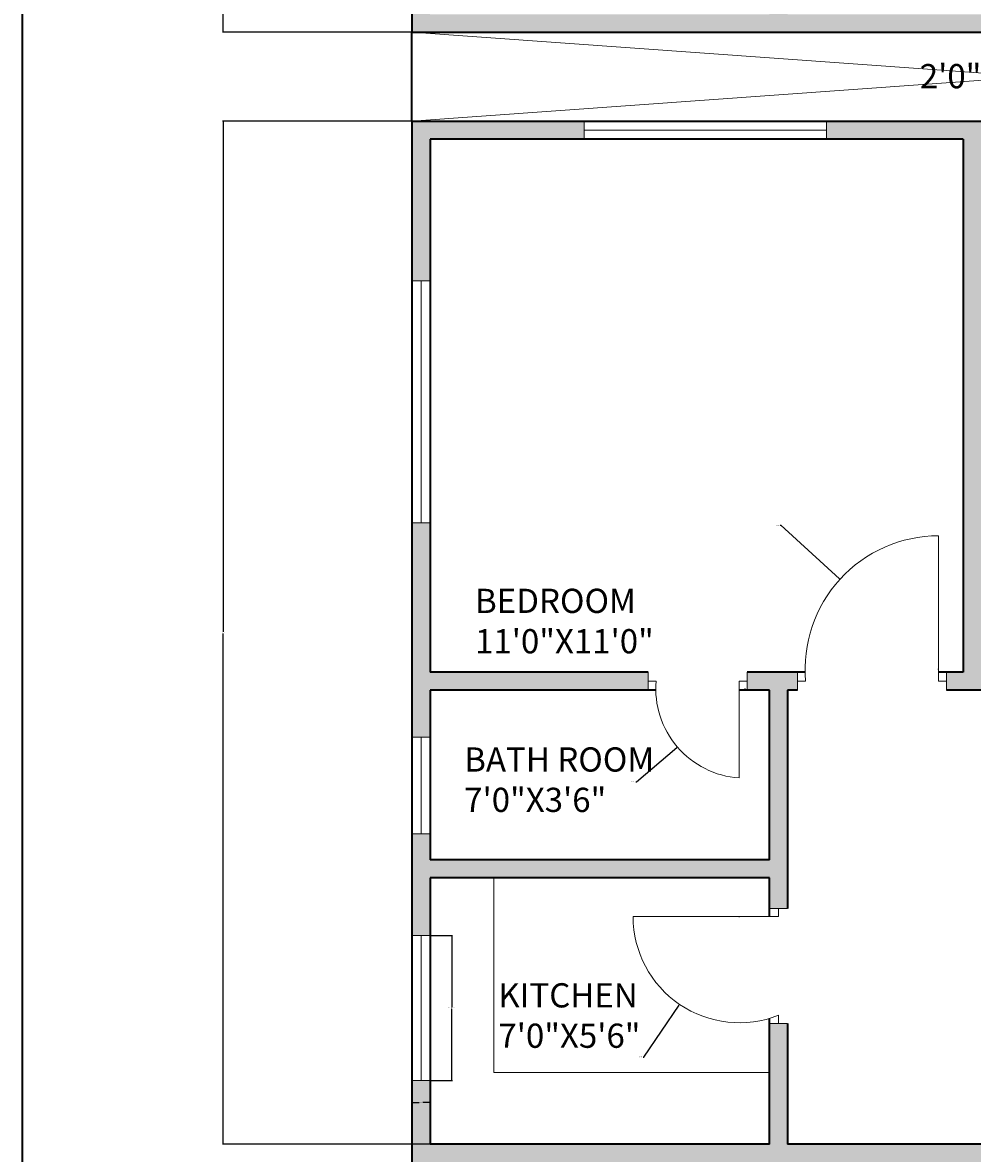
# Model space of a CAD drawing. Units: inches. Extents: x 2314 to 3223, y 1382 to 2735.
# Tile 6 of 14: x 2314 to 2549, y 1864 to 2144. Entities that reach past the tile are written whole.
import ezdxf

# ---------------------------------------------------------------- set-up
doc = ezdxf.new("R2010")
doc.units = ezdxf.units.IN
for name, color, linetype, lineweight in [('A-ANNO-DIMS', 2, 'Continuous', 18), ('A-ANNO-TTLB', 7, 'Continuous', 35), ('A-AREA-IDEN', 7, 'Continuous', 18), ('A-DOOR', 3, 'Continuous', 18), ('A-FLOR-FIXT', 8, 'Continuous', 18), ('A-FLOR-OPEN', 8, 'Continuous', 13), ('A-GLAZ', 4, 'Continuous', 18), ('A-WALL', 7, 'Continuous', 35)]:
    doc.layers.add(name, color=color, linetype=linetype, lineweight=lineweight)
doc.layers.add('A-WALL-PATT', color=251, linetype='Continuous', lineweight=13, true_color=0x636466)
doc.styles.get("Standard").update_dxf_attribs({"font": 'arial.ttf'})
doc.dimstyles.get("Standard").update_dxf_attribs({"dimtxt": 0.18, "dimasz": 0.18, "dimexe": 0.18, "dimexo": 0.0625, "dimgap": 0.09, "dimtad": 0, "dimtih": 1, "dimtoh": 1, "dimdec": 4, "dimzin": 0, "dimdsep": 46, "dimtxsty": 'Standard', "dimcen": 0.09, "dimadec": 0, "dimazin": 0, "dimtfac": 1, "dimtdec": 4, "dimtofl": 0, "dimtmove": 0, "dimatfit": 3, "dimfxl": 1, "dimtolj": 1, "dimtzin": 0, "dimarcsym": 0})

# ---------------------------------------------------------------- blocks, each defined once
blk = doc.blocks.new('WIN-PLAN-24-ALT')
for p, q in [((4.5, 24), (0, 24)), ((0, 24), (2.25, 24)), ((2.25, 24), (2.25, 0)), ((2.25, 0), (0, 0)), ((0, 0), (4.5, 0))]:
    blk.add_line(p, q)
blk = doc.blocks.new('WIN-PLAN-60')
for p, q in [((0, 4.5), (0, 0)), ((60, 2.25), (60, 4.5)), ((60, 4.5), (60, 0)), ((0, 0), (0, 2.25)), ((0, 2.25), (60, 2.25))]:
    blk.add_line(p, q)
blk = doc.blocks.new('WIN-PLAN-36')
for p, q in [((0, 36), (4.5, 36)), ((4.5, 36), (2.25, 36)), ((2.25, 36), (2.25, 0)), ((2.25, 0), (0, 0)), ((0, 0), (4.5, 0))]:
    blk.add_line(p, q)
blk = doc.blocks.new('*D15')
at = {"layer": 'A-ANNO-DIMS', "color": 0, "lineweight": -2, "transparency": 16777216}
for p, q in [((2414.96, 1918.15), (2420.47, 1918.15)), ((2420.29, 1917.97), (2420.29, 1900.33)), ((2420.29, 1882.33), (2420.29, 1899.97)), ((2414.96, 1882.15), (2420.47, 1882.15))]:
    blk.add_line(p, q, dxfattribs=at)
at = {"layer": 'A-ANNO-DIMS', "color": 0, "transparency": 16777216}
for points in [[(2420.26, 1917.97), (2420.32, 1917.97), (2420.29, 1918.15)], [(2420.26, 1882.33), (2420.32, 1882.33), (2420.29, 1882.15)]]:
    blk.add_solid(points, dxfattribs=at)
at = {"layer": 'Defpoints', "color": 0, "transparency": 16777216}
for p in [(2414.89, 1918.15), (2414.89, 1882.15), (2420.29, 1882.15)]:
    blk.add_point(p, dxfattribs=at)
at = {"layer": 'A-ANNO-DIMS', "color": 0, "transparency": 16777216, "insert": (2420.29, 1900.15), "char_height": 0.18, "attachment_point": 5}
blk.add_mtext('\\A1;WINDOW 36 TYP.', dxfattribs=at)
blk = doc.blocks.new('*D16')
at = {"layer": 'A-ANNO-DIMS', "color": 0, "lineweight": -2, "transparency": 16777216}
for p, q in [((2410.39, 1882.09), (2410.39, 1876.57)), ((2414.89, 1882.09), (2414.89, 1876.57)), ((2410.57, 1876.75), (2412.18, 1876.75)), ((2414.71, 1876.75), (2413.1, 1876.75))]:
    blk.add_line(p, q, dxfattribs=at)
at = {"layer": 'A-ANNO-DIMS', "color": 0, "transparency": 16777216}
for points in [[(2410.57, 1876.78), (2410.57, 1876.72), (2410.39, 1876.75)], [(2414.71, 1876.78), (2414.71, 1876.72), (2414.89, 1876.75)]]:
    blk.add_solid(points, dxfattribs=at)
at = {"layer": 'Defpoints', "color": 0, "transparency": 16777216}
for p in [(2410.39, 1882.15), (2414.89, 1882.15), (2410.39, 1876.75)]:
    blk.add_point(p, dxfattribs=at)
at = {"layer": 'A-ANNO-DIMS', "color": 0, "transparency": 16777216, "insert": (2412.64, 1876.75), "char_height": 0.18, "attachment_point": 5}
blk.add_mtext('\\A1;5 TYP.', dxfattribs=at)
blk = doc.blocks.new('*D33')
at = {"layer": 'A-ANNO-DIMS', "color": 0, "lineweight": -2, "transparency": 16777216}
for p, q in [((2410.33, 2119.88), (2363.51, 2119.88)), ((2363.69, 2119.7), (2363.69, 1993.32)), ((2363.69, 1866.56), (2363.69, 1992.95)), ((2414.83, 1866.38), (2363.51, 1866.38))]:
    blk.add_line(p, q, dxfattribs=at)
at = {"layer": 'A-ANNO-DIMS', "color": 0, "transparency": 16777216}
for points in [[(2363.66, 2119.7), (2363.72, 2119.7), (2363.69, 2119.88)], [(2363.66, 1866.56), (2363.72, 1866.56), (2363.69, 1866.38)]]:
    blk.add_solid(points, dxfattribs=at)
at = {"layer": 'Defpoints', "color": 0, "transparency": 16777216}
for p in [(2363.69, 2119.88), (2410.39, 2119.88), (2414.89, 1866.38)]:
    blk.add_point(p, dxfattribs=at)
at = {"layer": 'A-ANNO-DIMS', "color": 0, "transparency": 16777216, "insert": (2363.69, 1993.13), "char_height": 0.18, "attachment_point": 5}
blk.add_mtext('\\A1;253.5', dxfattribs=at)
blk = doc.blocks.new('*D34')
at = {"layer": 'A-ANNO-DIMS', "color": 0, "lineweight": -2, "transparency": 16777216}
for p, q in [((2410.33, 2381.78), (2363.51, 2381.78)), ((2363.69, 2381.6), (2363.69, 2262.02)), ((2363.69, 2142.06), (2363.69, 2261.65)), ((2410.33, 2141.88), (2363.51, 2141.88))]:
    blk.add_line(p, q, dxfattribs=at)
at = {"layer": 'A-ANNO-DIMS', "color": 0, "transparency": 16777216}
for points in [[(2363.66, 2381.6), (2363.72, 2381.6), (2363.69, 2381.78)], [(2363.66, 2142.06), (2363.72, 2142.06), (2363.69, 2141.88)]]:
    blk.add_solid(points, dxfattribs=at)
at = {"layer": 'Defpoints', "color": 0, "transparency": 16777216}
for p in [(2363.69, 2381.78), (2410.39, 2381.78), (2410.39, 2141.88)]:
    blk.add_point(p, dxfattribs=at)
at = {"layer": 'A-ANNO-DIMS', "color": 0, "transparency": 16777216, "insert": (2363.69, 2261.83), "char_height": 0.18, "attachment_point": 5}
blk.add_mtext('\\A1;239.9', dxfattribs=at)
blk = doc.blocks.new('*D65')
at = {"layer": 'A-ANNO-DIMS', "color": 0, "lineweight": -2, "transparency": 16777216}
for p, q in [((2501.56, 2019.75), (2501.74, 2019.75)), ((2501.74, 2019.75), (2516.24, 2006.51)), ((2540.66, 1984.11), (2540.84, 1984.11)), ((2540.75, 1984.02), (2540.75, 1984.2))]:
    blk.add_line(p, q, dxfattribs=at)
at = {"layer": 'A-ANNO-DIMS', "color": 0, "transparency": 16777216}
blk.add_solid([(2516.26, 2006.53), (2516.22, 2006.48), (2516.37, 2006.38)], dxfattribs=at)
at = {"layer": 'Defpoints', "color": 0, "transparency": 16777216}
for p in [(2516.37, 2006.38), (2540.75, 1984.11)]:
    blk.add_point(p, dxfattribs=at)
at = {"layer": 'A-ANNO-DIMS', "color": 0, "transparency": 16777216, "insert": (2501.08, 2019.75), "char_height": 0.18, "attachment_point": 5}
blk.add_mtext('\\A1;R33.03', dxfattribs=at)
blk = doc.blocks.new('*D78')
at = {"layer": 'A-ANNO-DIMS', "color": 0, "lineweight": -2, "transparency": 16777216}
for p, q in [((2491.35, 1922.79), (2491.53, 1922.79)), ((2491.44, 1922.7), (2491.44, 1922.88)), ((2467.81, 1887.98), (2476.57, 1900.88)), ((2467.63, 1887.98), (2467.81, 1887.98))]:
    blk.add_line(p, q, dxfattribs=at)
at = {"layer": 'A-ANNO-DIMS', "color": 0, "transparency": 16777216}
blk.add_solid([(2476.54, 1900.9), (2476.59, 1900.87), (2476.67, 1901.03)], dxfattribs=at)
at = {"layer": 'Defpoints', "color": 0, "transparency": 16777216}
for p in [(2491.44, 1922.79), (2476.67, 1901.03)]:
    blk.add_point(p, dxfattribs=at)
at = {"layer": 'A-ANNO-DIMS', "color": 0, "transparency": 16777216, "insert": (2467.08, 1887.98), "char_height": 0.18, "attachment_point": 5}
blk.add_mtext('\\A1;R26.296', dxfattribs=at)
blk = doc.blocks.new('*D84')
at = {"layer": 'A-ANNO-DIMS', "color": 0, "lineweight": -2, "transparency": 16777216}
for p, q in [((2492.81, 1979.22), (2492.99, 1979.22)), ((2492.9, 1979.13), (2492.9, 1979.31)), ((2465.98, 1956.2), (2475.94, 1964.71)), ((2465.8, 1956.2), (2465.98, 1956.2))]:
    blk.add_line(p, q, dxfattribs=at)
at = {"layer": 'A-ANNO-DIMS', "color": 0, "transparency": 16777216}
blk.add_solid([(2475.92, 1964.74), (2475.96, 1964.69), (2476.08, 1964.83)], dxfattribs=at)
at = {"layer": 'Defpoints', "color": 0, "transparency": 16777216}
for p in [(2492.9, 1979.22), (2476.08, 1964.83)]:
    blk.add_point(p, dxfattribs=at)
at = {"layer": 'A-ANNO-DIMS', "color": 0, "transparency": 16777216, "insert": (2465.25, 1956.2), "char_height": 0.18, "attachment_point": 5}
blk.add_mtext('\\A1;R22.137', dxfattribs=at)

msp = doc.modelspace()

# ---------------------------------------------------------------- hatches: boundary and pattern name
at = {"layer": 'A-WALL-PATT'}
h = msp.add_hatch(color=256, dxfattribs=at)
h.dxf.hatch_style = 1
h.paths.add_polyline_path([(2443.3302, 2379.5332), (2443.3302, 2381.7832), (2410.3927, 2381.7832), (2410.3927, 2336.7008), (2414.8927, 2336.7008), (2414.8927, 2377.2832), (2443.3302, 2377.2832)])
h.paths.add_polyline_path([(2561.3645, 2379.5332), (2561.3645, 2381.7832), (2503.3302, 2381.7832), (2503.3302, 2377.2832), (2546.8927, 2377.2832), (2546.8927, 2245.2832), (2541.8787, 2245.2832), (2541.8787, 2240.7832), (2551.3927, 2240.7832), (2551.3927, 2377.2832), (2561.3645, 2377.2832)])
h.paths.add_polyline_path([(2656.0607, 2381.7832), (2597.3645, 2381.7832), (2597.3645, 2377.2832), (2617.3927, 2377.2832), (2617.3927, 2257.2832), (2584.2532, 2257.2832), (2584.2532, 2252.7832), (2625.8528, 2252.7832), (2625.8528, 2255.0332), (2625.8528, 2257.2832), (2621.8927, 2257.2832), (2621.8927, 2377.2832), (2656.0607, 2377.2832), (2656.0607, 2379.5332)])
h.paths.add_polyline_path([(2807.3418, 2381.7832), (2716.0607, 2381.7832), (2716.0607, 2377.2832), (2765.8927, 2377.2832), (2765.8927, 2257.2832), (2661.6935, 2257.2832), (2661.6935, 2252.7832), (2765.8927, 2252.7832), (2765.8927, 2146.2832), (2760.9259, 2146.2832), (2760.9259, 2141.8832), (2775.7119, 2141.8832), (2775.7119, 2146.2832), (2770.3927, 2146.2832), (2770.3927, 2252.7832), (2877.684, 2252.7832), (2877.684, 2255.0332), (2877.684, 2257.2832), (2770.3927, 2257.2832), (2770.3927, 2377.2832), (2807.3418, 2377.2832), (2807.3418, 2379.5332)])
h.paths.add_polyline_path([(2937.2118, 2381.7832), (2867.3418, 2381.7832), (2867.3418, 2377.2832), (2914.3927, 2377.2832), (2914.3927, 2257.2832), (2908.4124, 2257.2832), (2908.4124, 2252.7832), (2960.6432, 2252.7832), (2960.6432, 2255.0332), (2960.6432, 2257.2832), (2918.8927, 2257.2832), (2918.8927, 2377.2832), (2937.2118, 2377.2832)])
h.paths.add_polyline_path([(3022.1601, 2381.7832), (2973.2118, 2381.7832), (2973.2118, 2379.5332), (2973.2118, 2377.2832), (2984.8927, 2377.2832), (2984.8927, 2257.2832), (2980.0601, 2257.2832), (2980.0601, 2252.7832), (2984.8927, 2252.7832), (2984.8927, 2240.7832), (2995.668, 2240.7832), (2995.668, 2243.0332), (2995.668, 2245.2832), (2989.3927, 2245.2832), (2989.3927, 2377.2832), (3022.1601, 2377.2832), (3022.1601, 2379.5332)])
h.paths.add_polyline_path([(3125.8927, 2381.7832), (3082.1601, 2381.7832), (3082.1601, 2377.2832), (3121.3927, 2377.2832), (3121.3927, 2334.7388), (3125.8927, 2334.7388)])
h.paths.add_polyline_path([(3125.8927, 2274.7388), (3121.3927, 2274.7388), (3121.3927, 2245.2832), (3066.4832, 2245.2832), (3066.4832, 2240.7832), (3121.3927, 2240.7832), (3121.3927, 2232.1868), (3125.8927, 2232.1868)])
h.paths.add_polyline_path([(3125.8927, 2208.1868), (3121.3927, 2208.1868), (3121.3927, 2198.7832), (3037.3927, 2198.7832), (3037.3927, 2240.7832), (3041.2694, 2240.7832), (3041.2694, 2243.0332), (3041.2694, 2245.2832), (3026.8205, 2245.2832), (3026.8205, 2240.7832), (3032.8927, 2240.7832), (3032.8927, 2190.4022), (3037.3927, 2190.4022), (3037.3927, 2194.2832), (3121.3927, 2194.2832), (3121.3927, 2182.1835), (3125.8927, 2182.1835)])
h.paths.add_polyline_path([(3125.8927, 2158.1835), (3121.3927, 2158.1835), (3121.3927, 2146.2832), (3037.3927, 2146.2832), (3037.3927, 2169.3726), (3035.1427, 2169.3726), (3032.8927, 2169.3726), (3032.8927, 2146.2832), (2812.7301, 2146.2832), (2812.7301, 2144.0832), (2812.7301, 2141.8832), (2818.3927, 2141.8832), (2818.3927, 1970.1316), (2822.8927, 1970.1316), (2822.8927, 1978.8832), (2903.9846, 1978.8832), (2903.9846, 1981.1332), (2903.9846, 1983.3832), (2822.8927, 1983.3832), (2822.8927, 2115.3832), (2851.7162, 2115.3832), (2851.7162, 2117.6332), (2851.7162, 2119.8832), (2822.8927, 2119.8832), (2822.8927, 2141.8832), (3125.8927, 2141.8832)])
h.paths.add_polyline_path([(3125.8927, 2119.8832), (3081.193, 2119.8832), (3081.193, 2115.3832), (3121.3927, 2115.3832), (3121.3927, 2071.8188), (3125.8927, 2071.8188)], flags=17)
h.paths.add_polyline_path([(2989.3927, 2115.3832), (3021.193, 2115.3832), (3021.193, 2117.6332), (3021.193, 2119.8832), (2979.123, 2119.8832), (2979.123, 2115.3832), (2984.8927, 2115.3832), (2984.8927, 2019.3832), (2981.9225, 2019.3832), (2981.9225, 2014.8832), (2984.8927, 2014.8832), (2984.8927, 1983.3832), (2984.8927, 1978.8832), (2989.3927, 1978.8832), (2989.3927, 1983.3832)], flags=17)
h.paths.add_polyline_path([(2947.3927, 2115.3832), (2955.123, 2115.3832), (2955.123, 2117.6332), (2955.123, 2119.8832), (2911.7162, 2119.8832), (2911.7162, 2115.3832), (2942.8927, 2115.3832), (2942.8927, 1983.3832), (2936.7017, 1983.3832), (2936.7017, 1978.8832), (2947.3927, 1978.8832), (2947.3927, 1983.3832), (2947.3927, 2014.8832), (2960.7167, 2014.8832), (2960.7167, 2017.1332), (2960.7167, 2019.3832), (2947.3927, 2019.3832)], flags=17)
h.paths.add_polyline_path([(3037.3927, 1978.8832), (3041.8276, 1978.8832), (3041.8276, 1981.1332), (3041.8276, 1983.3832), (3025.477, 1983.3832), (3025.477, 1978.8832), (3032.8927, 1978.8832), (3032.8927, 1927.1259), (3035.1427, 1927.1259), (3037.3927, 1927.1259)])
h.paths.add_polyline_path([(3125.8927, 2011.8188), (3123.6427, 2011.8188), (3121.3927, 2011.8188), (3121.3927, 1983.3832), (3065, 1983.3832), (3065, 1978.8832), (3121.3927, 1978.8832), (3121.3927, 1970.5932), (3125.8927, 1970.5932)], flags=17)
h.paths.add_polyline_path([(2994.2341, 1983.3832), (2989.3927, 1983.3832), (2989.3927, 1978.8832), (2994.2341, 1978.8832), (2994.2341, 1981.1332)], flags=16)
h.paths.add_polyline_path([(3125.8927, 1946.5932), (3121.3927, 1946.5932), (3121.3927, 1936.8832), (3037.3927, 1936.8832), (3037.3927, 1932.3832), (3121.3927, 1932.3832), (3121.3927, 1919.825), (3125.8927, 1919.825)])
h.paths.add_polyline_path([(3125.8927, 1883.825), (3121.3927, 1883.825), (3121.3927, 1866.3832), (3037.3927, 1866.3832), (3037.3927, 1899.0954), (3035.1427, 1899.0954), (3032.8927, 1899.0954), (3032.8927, 1866.3832), (2822.8927, 1866.3832), (2822.8927, 1938.7212), (2820.6427, 1938.7212), (2818.3927, 1938.7212), (2818.3927, 1786.9239), (2822.8927, 1786.9239), (2822.8927, 1861.8832), (3032.8927, 1861.8832), (3032.8927, 1825.1023), (3037.3927, 1825.1023), (3037.3927, 1861.8832), (3121.3927, 1861.8832), (3121.3927, 1844.6765), (3125.8927, 1844.6765)])
h.paths.add_polyline_path([(3125.8927, 1808.6765), (3121.3927, 1808.6765), (3121.3927, 1795.8832), (3037.3927, 1795.8832), (3037.3927, 1799.4755), (3032.8927, 1799.4755), (3032.8927, 1749.3832), (3026.5034, 1749.3832), (3026.5034, 1744.8832), (3032.8927, 1744.8832), (3034.9255, 1744.8832), (3043.1326, 1744.8832), (3043.1326, 1747.1332), (3043.1326, 1749.3832), (3037.3927, 1749.3832), (3037.3927, 1791.3832), (3121.3927, 1791.3832), (3121.3927, 1783.3103), (3125.8927, 1783.3103)])
h.paths.add_polyline_path([(3125.8927, 1759.3103), (3121.3927, 1759.3103), (3121.3927, 1749.3832), (3065.1845, 1749.3832), (3065.1845, 1744.8832), (3121.3927, 1744.8832), (3121.3927, 1709.3573), (3125.8927, 1709.3573)])
h.paths.add_polyline_path([(3125.8927, 1649.3573), (3121.3927, 1649.3573), (3121.3927, 1612.8832), (3095.116, 1612.8832), (3095.116, 1608.3832), (3125.8927, 1608.3832)])
h.paths.add_polyline_path([(3035.116, 1612.8832), (2993.8927, 1612.8832), (2993.8927, 1744.8832), (2998.7409, 1744.8832), (2998.7409, 1749.3832), (2989.3927, 1749.3832), (2989.3927, 1744.8832), (2989.3927, 1701.3832), (2972.8226, 1701.3832), (2972.8226, 1696.8832), (2989.3927, 1696.8832), (2989.3927, 1612.8832), (2978.2225, 1612.8832), (2978.2225, 1608.3832), (3035.116, 1608.3832), (3035.116, 1610.6332)])
h.paths.add_polyline_path([(2947.3927, 1696.8832), (2950.7566, 1696.8832), (2950.7566, 1699.1332), (2950.7566, 1701.3832), (2947.3927, 1701.3832), (2947.3927, 1744.8832), (2947.3927, 1749.3832), (2937.649, 1749.3832), (2937.649, 1744.8832), (2942.8927, 1744.8832), (2942.8927, 1612.8832), (2907.783, 1612.8832), (2907.783, 1608.3832), (2954.2225, 1608.3832), (2954.2225, 1610.6332), (2954.2225, 1612.8832), (2947.3927, 1612.8832)])
h.paths.add_polyline_path([(2822.8927, 1744.8832), (2905.3491, 1744.8832), (2905.3491, 1747.1332), (2905.3491, 1749.3832), (2822.8927, 1749.3832), (2822.8927, 1756.9185), (2818.3927, 1756.9185), (2818.3927, 1612.8832), (2818.3927, 1569.1205), (2722.3927, 1569.1205), (2722.3927, 1612.8832), (2722.3927, 1756.9185), (2717.8927, 1756.9185), (2717.8927, 1750.0143), (2633.6297, 1750.0143), (2633.6437, 1745.2665), (2717.8927, 1745.5143), (2717.8927, 1612.8832), (2689.8467, 1612.8832), (2689.8467, 1608.3832), (2717.8927, 1608.3832), (2717.8927, 1564.6205), (2722.3927, 1564.6205), (2822.8927, 1564.6205), (2822.8927, 1569.1205), (2822.8927, 1608.3832), (2847.783, 1608.3832), (2847.783, 1610.6332), (2847.783, 1612.8832), (2822.8927, 1612.8832)])
h.paths.add_polyline_path([(2629.8467, 1612.8832), (2597.8927, 1612.8832), (2597.8927, 1744.8832), (2597.8927, 1745.1613), (2601.5887, 1745.1721), (2601.5816, 1747.5932), (2601.5745, 1750.0143), (2593.3927, 1750.0143), (2593.3927, 1744.8832), (2593.3927, 1713.3832), (2589.7588, 1713.3832), (2589.7588, 1708.8832), (2593.3927, 1708.8832), (2593.3927, 1612.8832), (2582.3793, 1612.8832), (2582.3793, 1608.3832), (2629.8467, 1608.3832), (2629.8467, 1610.6332)])
h.paths.add_polyline_path([(2551.3927, 1708.8832), (2567.6776, 1708.8832), (2567.6776, 1711.1332), (2567.6776, 1713.3832), (2551.3927, 1713.3832), (2551.3927, 1744.8832), (2551.3927, 1750.0143), (2543.5657, 1750.0143), (2543.5657, 1747.5079), (2543.5657, 1745.0014), (2546.8927, 1745.0112), (2546.8927, 1744.8832), (2546.8927, 1612.8832), (2502.9339, 1612.8832), (2502.9339, 1608.3832), (2558.3793, 1608.3832), (2558.3793, 1610.6332), (2558.3793, 1612.8832), (2551.3927, 1612.8832)])
h.paths.add_polyline_path([(2414.8927, 1656.2547), (2410.3927, 1656.2547), (2410.3927, 1608.3832), (2442.9339, 1608.3832), (2442.9339, 1610.6332), (2442.9339, 1612.8832), (2414.8927, 1612.8832)])
h.paths.add_polyline_path([(2414.8927, 1744.8832), (2468.8906, 1744.8832), (2468.8906, 1747.1332), (2468.8906, 1749.3832), (2414.8927, 1749.3832), (2414.8927, 1757.7622), (2410.3927, 1757.7622), (2410.3927, 1716.2547), (2414.8927, 1716.2547)])
h.paths.add_polyline_path([(2414.8927, 1791.3832), (2498.8927, 1791.3832), (2498.8927, 1749.3832), (2492.9799, 1749.3832), (2492.9799, 1744.8832), (2498.8927, 1744.8832), (2503.3927, 1744.8832), (2508.0135, 1744.8968), (2508.0059, 1747.4556), (2507.9984, 1750.0143), (2503.3927, 1750.0143), (2503.3927, 1802.6362), (2501.1427, 1802.6362), (2498.8927, 1802.6362), (2498.8927, 1795.8832), (2414.8927, 1795.8832), (2414.8927, 1808.0943), (2410.3927, 1808.0943), (2410.3927, 1781.7622), (2414.8927, 1781.7622)])
h.paths.add_polyline_path([(2722.3927, 1937.589), (2720.1427, 1937.589), (2717.8927, 1937.589), (2717.8927, 1866.3832), (2503.3927, 1866.3832), (2503.3927, 1896.3484), (2498.8927, 1896.3484), (2498.8927, 1866.3832), (2414.8927, 1866.3832), (2414.8927, 1882.1496), (2410.3927, 1882.1496), (2410.3927, 1844.0943), (2414.8927, 1844.0943), (2414.8927, 1861.8832), (2498.8927, 1861.8832), (2498.8927, 1831.4783), (2501.1427, 1831.4783), (2503.3927, 1831.4783), (2503.3927, 1861.8832), (2717.8927, 1861.8832), (2717.8927, 1786.9239), (2722.3927, 1786.9239)])
h.paths.add_polyline_path([(2414.8927, 1932.3832), (2498.8927, 1932.3832), (2498.8927, 1924.7883), (2503.3927, 1924.7883), (2503.3927, 1978.8832), (2505.8599, 1978.8832), (2505.8599, 1981.1332), (2505.8599, 1983.3832), (2493.3697, 1983.3832), (2493.3697, 1978.8832), (2498.8927, 1978.8832), (2498.8927, 1936.8832), (2414.8927, 1936.8832), (2414.8927, 1943.2834), (2410.3927, 1943.2834), (2410.3927, 1918.1496), (2414.8927, 1918.1496)])
h.paths.add_polyline_path([(2414.8927, 2020.3133), (2412.6427, 2020.3133), (2410.3927, 2020.3133), (2410.3927, 1967.2834), (2414.8927, 1967.2834), (2414.8927, 1978.8832), (2468.8513, 1978.8832), (2468.8513, 1981.1332), (2468.8513, 1983.3832), (2414.8927, 1983.3832)])
h.paths.add_polyline_path([(2414.8927, 2115.3832), (2453.004, 2115.3832), (2453.004, 2117.6332), (2453.004, 2119.8832), (2410.3927, 2119.8832), (2410.3927, 2080.3133), (2414.8927, 2080.3133)], flags=17)
h.paths.add_polyline_path([(2559.0969, 2117.6332), (2559.0969, 2119.8832), (2513.004, 2119.8832), (2513.004, 2115.3832), (2546.8927, 2115.3832), (2546.8927, 1983.3832), (2542.7531, 1983.3832), (2542.7531, 1978.8832), (2551.3927, 1978.8832), (2551.3927, 2014.8832), (2570.3098, 2014.8832), (2570.3098, 2017.1332), (2570.3098, 2019.3832), (2551.3927, 2019.3832), (2551.3927, 2115.3832), (2559.0969, 2115.3832)], flags=17)
h.paths.add_polyline_path([(2628.5073, 2117.6332), (2628.5073, 2119.8832), (2583.0969, 2119.8832), (2583.0969, 2115.3832), (2593.3927, 2115.3832), (2593.3927, 2019.3832), (2590.2108, 2019.3832), (2590.2108, 2014.8832), (2593.3927, 2014.8832), (2593.3927, 1978.8832), (2601.5907, 1978.8832), (2601.5907, 1981.1332), (2601.5907, 1983.3832), (2597.8927, 1983.3832), (2597.8927, 2115.3832), (2628.5073, 2115.3832)], flags=17)
h.paths.add_polyline_path([(2722.3927, 2141.8832), (2726.9871, 2141.8832), (2726.9871, 2144.2705), (2726.9871, 2146.2832), (2503.3927, 2146.2832), (2503.3927, 2168.2161), (2501.1427, 2168.2161), (2498.8927, 2168.2161), (2498.8927, 2146.2832), (2414.8927, 2146.2832), (2414.8927, 2156.5041), (2410.3927, 2156.5041), (2410.3927, 2141.8832), (2717.8927, 2141.8832), (2717.8927, 2119.8832), (2688.5073, 2119.8832), (2688.5073, 2115.3832), (2717.8927, 2115.3832), (2717.8927, 1983.3832), (2633.2454, 1983.3832), (2633.2454, 1978.8832), (2717.8927, 1978.8832), (2717.8927, 1970.1316), (2720.1427, 1970.1316), (2722.3927, 1970.1316)])
h.paths.add_polyline_path([(2557.3704, 1462.9278), (2940.0934, 1462.9278), (2940.0934, 1512.3848), (2557.3704, 1512.3848)], flags=9)
h.paths.add_polyline_path([(2846.2527, 1703.1384), (2892.8612, 1703.1384), (2892.8612, 1725.5272), (2846.2527, 1725.5272)], flags=25)
h.paths.add_polyline_path([(2885.6102, 1812.1147), (2946.1505, 1812.1147), (2946.1505, 1834.5035), (2885.6102, 1834.5035)], flags=25)
h.paths.add_polyline_path([(2885.6102, 1884.183), (2946.1505, 1884.183), (2946.1505, 1906.5718), (2885.6102, 1906.5718)], flags=25)
h.paths.add_polyline_path([(3066.365, 1705.5431), (3112.9735, 1705.5431), (3112.9735, 1727.9319), (3066.365, 1727.9319)], flags=9)
h.paths.add_polyline_path([(3061.8255, 1887.7513), (3101.6154, 1887.7513), (3101.6154, 1910.1401), (3061.8255, 1910.1401)], flags=25)
h.paths.add_polyline_path([(3063.3679, 1816.2121), (3103.1578, 1816.2121), (3103.1578, 1838.6009), (3063.3679, 1838.6009)], flags=25)
h.paths.add_polyline_path([(3053.3743, 1768.416), (3107.1329, 1768.416), (3107.1329, 1790.8048), (3053.3743, 1790.8048)], flags=25)
h.paths.add_polyline_path([(3061.6068, 1943.822), (3115.3653, 1943.822), (3115.3653, 1966.2109), (3061.6068, 1966.2109)], flags=9)
h.paths.add_polyline_path([(2745.0978, 1763.6604), (2797.9354, 1763.6604), (2797.9354, 1776.0247), (2745.0978, 1776.0247)], flags=9)
h.paths.add_polyline_path([(2574.2135, 1819.2586), (2634.7538, 1819.2586), (2634.7538, 1841.6474), (2574.2135, 1841.6474)], flags=25)
h.paths.add_polyline_path([(2574.2135, 1891.3269), (2634.7538, 1891.3269), (2634.7538, 1913.7157), (2574.2135, 1913.7157)], flags=25)
h.paths.add_polyline_path([(2638.4466, 1702.43), (2685.0551, 1702.43), (2685.0551, 1724.8188), (2638.4466, 1724.8188)], flags=25)
h.paths.add_polyline_path([(2435.9715, 1697.1215), (2482.5799, 1697.1215), (2482.5799, 1719.5103), (2435.9715, 1719.5103)], flags=9)
h.paths.add_polyline_path([(2431.2046, 1893.7833), (2470.9945, 1893.7833), (2470.9945, 1916.1721), (2431.2046, 1916.1721)], flags=25)
h.paths.add_polyline_path([(2439.8144, 1817.2116), (2479.6043, 1817.2116), (2479.6043, 1839.6004), (2439.8144, 1839.6004)], flags=25)
h.paths.add_polyline_path([(2441.2607, 1753.0942), (2495.0192, 1753.0942), (2495.0192, 1775.483), (2441.2607, 1775.483)], flags=25)
h.paths.add_polyline_path([(2421.216, 1945.3109), (2474.9746, 1945.3109), (2474.9746, 1967.6997), (2421.216, 1967.6997)], flags=25)
h.paths.add_polyline_path([(2585.4464, 1627.5703), (2585.4464, 1679), (2563.0576, 1679), (2563.0576, 1627.5703)], flags=9)
h.paths.add_polyline_path([(2978.3497, 1618.7039), (2978.3497, 1670.1337), (2955.9609, 1670.1337), (2955.9609, 1618.7039)], flags=9)
h.paths.add_polyline_path([(2975.9502, 2041.7828), (2975.9502, 2093.2125), (2953.5614, 2093.2125), (2953.5614, 2041.7828)], flags=25)
h.paths.add_polyline_path([(2835.6537, 1989.2068), (2882.2621, 1989.2068), (2882.2621, 2011.5956), (2835.6537, 2011.5956)], flags=25)
h.paths.add_polyline_path([(2649.3769, 1997.5659), (2695.9853, 1997.5659), (2695.9853, 2019.9547), (2649.3769, 2019.9547)], flags=25)
h.paths.add_polyline_path([(2579.9087, 2040.3429), (2579.9087, 2091.7726), (2557.5198, 2091.7726), (2557.5198, 2040.3429)], flags=25)
h.paths.add_polyline_path([(2783.2404, 1883.1956), (2783.2404, 2067.1369), (2764.694, 2067.1369), (2764.694, 1883.1956)], flags=9)
h.paths.add_polyline_path([(3055.8435, 1993.5571), (3102.4519, 1993.5571), (3102.4519, 2015.9459), (3055.8435, 2015.9459)], flags=25)
h.paths.add_polyline_path([(2423.6009, 1984.6082), (2470.2094, 1984.6082), (2470.2094, 2006.997), (2423.6009, 2006.997)], flags=25)
h.paths.add_polyline_path([(2973.4115, 2123.1668), (3013.1319, 2123.1668), (3013.1319, 2135.531), (2973.4115, 2135.531)], flags=25)
h.paths.add_polyline_path([(2534.3846, 2124.6231), (2574.105, 2124.6231), (2574.105, 2136.9874), (2534.3846, 2136.9874)], flags=25)
h.paths.add_polyline_path([(2829.1368, 2188.1931), (2889.411, 2188.1931), (2889.411, 2210.5819), (2829.1368, 2210.5819)], flags=9)
h.paths.add_polyline_path([(2633.2547, 2185.0437), (2693.5289, 2185.0437), (2693.5289, 2207.4325), (2633.2547, 2207.4325)], flags=9)
h.paths.add_polyline_path([(2445.1812, 2167.0395), (2496.611, 2167.0395), (2496.611, 2189.4284), (2445.1812, 2189.4284)], flags=9)
h.paths.add_polyline_path([(2429.1678, 2194.5482), (2480.5975, 2194.5482), (2480.5975, 2216.937), (2429.1678, 2216.937)], flags=9)
h.paths.add_polyline_path([(3060.1138, 2158.1056), (3111.5436, 2158.1056), (3111.5436, 2180.4944), (3060.1138, 2180.4944)], flags=9)
h.paths.add_polyline_path([(3055.6824, 2201.2631), (3107.1122, 2201.2631), (3107.1122, 2223.652), (3055.6824, 2223.652)], flags=25)
h.paths.add_polyline_path([(3044.3482, 2257.7345), (3090.9567, 2257.7345), (3090.9567, 2280.1233), (3044.3482, 2280.1233)], flags=9)
h.paths.add_polyline_path([(2942.5437, 2306.9625), (2982.3336, 2306.9625), (2982.3336, 2329.3513), (2942.5437, 2329.3513)], flags=9)
h.paths.add_polyline_path([(2799.5865, 2259.1663), (2846.195, 2259.1663), (2846.195, 2281.5551), (2799.5865, 2281.5551)], flags=25)
h.paths.add_polyline_path([(2670.4998, 2261.1493), (2717.1082, 2261.1493), (2717.1082, 2283.5381), (2670.4998, 2283.5381)], flags=25)
h.paths.add_polyline_path([(2553.0333, 2302.7735), (2592.8232, 2302.7735), (2592.8232, 2325.1624), (2553.0333, 2325.1624)], flags=9)
h.paths.add_polyline_path([(2432.0288, 2268.6489), (2478.6372, 2268.6489), (2478.6372, 2291.0377), (2432.0288, 2291.0377)], flags=9)
h = msp.add_hatch(color=256, dxfattribs=at)
h.dxf.hatch_style = 1
h.paths.add_polyline_path([(2503.3927, 2240.7832), (2507.7952, 2240.7832), (2507.7952, 2245.2832), (2496.4262, 2245.2832), (2496.4262, 2243.0332), (2496.4262, 2240.7832), (2498.8927, 2240.7832), (2498.8927, 2198.7832), (2414.8927, 2198.7832), (2414.8927, 2206.5718), (2410.3927, 2206.5718), (2410.3927, 2180.5041), (2412.6427, 2180.5041), (2414.8927, 2180.5041), (2414.8927, 2194.2832), (2498.8927, 2194.2832), (2498.8927, 2191.0069), (2503.3927, 2191.0069)])
h.paths.add_polyline_path([(2414.8927, 2276.7008), (2410.3927, 2276.7008), (2410.3927, 2230.5718), (2414.8927, 2230.5718), (2414.8927, 2240.7832), (2474.2564, 2240.7832), (2474.2564, 2243.0332), (2474.2564, 2245.2832), (2414.8927, 2245.2832)])
h.paths.add_polyline_path([(2557.3704, 1462.9278), (2940.0934, 1462.9278), (2940.0934, 1512.3848), (2557.3704, 1512.3848)], flags=9)
h.paths.add_polyline_path([(2846.2527, 1703.1384), (2892.8612, 1703.1384), (2892.8612, 1725.5272), (2846.2527, 1725.5272)], flags=9)
h.paths.add_polyline_path([(2885.6102, 1812.1147), (2946.1505, 1812.1147), (2946.1505, 1834.5035), (2885.6102, 1834.5035)], flags=9)
h.paths.add_polyline_path([(2885.6102, 1884.183), (2946.1505, 1884.183), (2946.1505, 1906.5718), (2885.6102, 1906.5718)], flags=9)
h.paths.add_polyline_path([(3066.365, 1705.5431), (3112.9735, 1705.5431), (3112.9735, 1727.9319), (3066.365, 1727.9319)], flags=9)
h.paths.add_polyline_path([(3061.8255, 1887.7513), (3101.6154, 1887.7513), (3101.6154, 1910.1401), (3061.8255, 1910.1401)], flags=9)
h.paths.add_polyline_path([(3063.3679, 1816.2121), (3103.1578, 1816.2121), (3103.1578, 1838.6009), (3063.3679, 1838.6009)], flags=9)
h.paths.add_polyline_path([(3053.3743, 1768.416), (3107.1329, 1768.416), (3107.1329, 1790.8048), (3053.3743, 1790.8048)], flags=9)
h.paths.add_polyline_path([(3061.6068, 1943.822), (3115.3653, 1943.822), (3115.3653, 1966.2109), (3061.6068, 1966.2109)], flags=9)
h.paths.add_polyline_path([(2745.0978, 1763.6604), (2797.9354, 1763.6604), (2797.9354, 1776.0247), (2745.0978, 1776.0247)], flags=9)
h.paths.add_polyline_path([(2574.2135, 1819.2586), (2634.7538, 1819.2586), (2634.7538, 1841.6474), (2574.2135, 1841.6474)], flags=9)
h.paths.add_polyline_path([(2574.2135, 1891.3269), (2634.7538, 1891.3269), (2634.7538, 1913.7157), (2574.2135, 1913.7157)], flags=9)
h.paths.add_polyline_path([(2638.4466, 1702.43), (2685.0551, 1702.43), (2685.0551, 1724.8188), (2638.4466, 1724.8188)], flags=9)
h.paths.add_polyline_path([(2435.9715, 1697.1215), (2482.5799, 1697.1215), (2482.5799, 1719.5103), (2435.9715, 1719.5103)], flags=9)
h.paths.add_polyline_path([(2431.2046, 1893.7833), (2470.9945, 1893.7833), (2470.9945, 1916.1721), (2431.2046, 1916.1721)], flags=9)
h.paths.add_polyline_path([(2439.8144, 1817.2116), (2479.6043, 1817.2116), (2479.6043, 1839.6004), (2439.8144, 1839.6004)], flags=9)
h.paths.add_polyline_path([(2441.2607, 1753.0942), (2495.0192, 1753.0942), (2495.0192, 1775.483), (2441.2607, 1775.483)], flags=9)
h.paths.add_polyline_path([(2421.216, 1945.3109), (2474.9746, 1945.3109), (2474.9746, 1967.6997), (2421.216, 1967.6997)], flags=9)
h.paths.add_polyline_path([(2585.4464, 1627.5703), (2585.4464, 1679), (2563.0576, 1679), (2563.0576, 1627.5703)], flags=9)
h.paths.add_polyline_path([(2978.3497, 1618.7039), (2978.3497, 1670.1337), (2955.9609, 1670.1337), (2955.9609, 1618.7039)], flags=9)
h.paths.add_polyline_path([(2975.9502, 2041.7828), (2975.9502, 2093.2125), (2953.5614, 2093.2125), (2953.5614, 2041.7828)], flags=9)
h.paths.add_polyline_path([(2835.6537, 1989.2068), (2882.2621, 1989.2068), (2882.2621, 2011.5956), (2835.6537, 2011.5956)], flags=9)
h.paths.add_polyline_path([(2649.3769, 1997.5659), (2695.9853, 1997.5659), (2695.9853, 2019.9547), (2649.3769, 2019.9547)], flags=9)
h.paths.add_polyline_path([(2579.9087, 2040.3429), (2579.9087, 2091.7726), (2557.5198, 2091.7726), (2557.5198, 2040.3429)], flags=9)
h.paths.add_polyline_path([(2783.2404, 1883.1956), (2783.2404, 2067.1369), (2764.694, 2067.1369), (2764.694, 1883.1956)], flags=9)
h.paths.add_polyline_path([(3055.8435, 1993.5571), (3102.4519, 1993.5571), (3102.4519, 2015.9459), (3055.8435, 2015.9459)], flags=9)
h.paths.add_polyline_path([(2423.6009, 1984.6082), (2470.2094, 1984.6082), (2470.2094, 2006.997), (2423.6009, 2006.997)], flags=9)
h.paths.add_polyline_path([(2973.4115, 2123.1668), (3013.1319, 2123.1668), (3013.1319, 2135.531), (2973.4115, 2135.531)], flags=9)
h.paths.add_polyline_path([(2534.3846, 2124.6231), (2574.105, 2124.6231), (2574.105, 2136.9874), (2534.3846, 2136.9874)], flags=9)
h.paths.add_polyline_path([(2829.1368, 2188.1931), (2889.411, 2188.1931), (2889.411, 2210.5819), (2829.1368, 2210.5819)], flags=9)
h.paths.add_polyline_path([(2633.2547, 2185.0437), (2693.5289, 2185.0437), (2693.5289, 2207.4325), (2633.2547, 2207.4325)], flags=9)
h.paths.add_polyline_path([(2445.1812, 2167.0395), (2496.611, 2167.0395), (2496.611, 2189.4284), (2445.1812, 2189.4284)], flags=9)
h.paths.add_polyline_path([(2429.1678, 2208.3022), (2480.5975, 2208.3022), (2480.5975, 2230.691), (2429.1678, 2230.691)], flags=25)
h.paths.add_polyline_path([(3060.1138, 2158.1056), (3111.5436, 2158.1056), (3111.5436, 2180.4944), (3060.1138, 2180.4944)], flags=9)
h.paths.add_polyline_path([(3055.6824, 2201.2631), (3107.1122, 2201.2631), (3107.1122, 2223.652), (3055.6824, 2223.652)], flags=9)
h.paths.add_polyline_path([(3044.3482, 2257.7345), (3090.9567, 2257.7345), (3090.9567, 2280.1233), (3044.3482, 2280.1233)], flags=9)
h.paths.add_polyline_path([(2942.5437, 2306.9625), (2982.3336, 2306.9625), (2982.3336, 2329.3513), (2942.5437, 2329.3513)], flags=9)
h.paths.add_polyline_path([(2799.5865, 2259.1663), (2846.195, 2259.1663), (2846.195, 2281.5551), (2799.5865, 2281.5551)], flags=9)
h.paths.add_polyline_path([(2670.4998, 2261.1493), (2717.1082, 2261.1493), (2717.1082, 2283.5381), (2670.4998, 2283.5381)], flags=9)
h.paths.add_polyline_path([(2553.0333, 2302.7735), (2592.8232, 2302.7735), (2592.8232, 2325.1624), (2553.0333, 2325.1624)], flags=9)
h.paths.add_polyline_path([(2432.0288, 2268.6489), (2478.6372, 2268.6489), (2478.6372, 2291.0377), (2432.0288, 2291.0377)], flags=9)

# ---------------------------------------------------------------- linework, layer by layer
at = {"layer": 'A-ANNO-TTLB'}
msp.add_lwpolyline([(2314.008, 2735.417), (3222.6676, 2735.417), (3222.6676, 1382.0876), (2314.008, 1382.0876)], close=True, dxfattribs=at)
at = {"layer": 'A-DOOR'}
for p, q in [((2540.7531, 1981.1332), (2540.7531, 2017.1332)), ((2468.8513, 1983.3832), (2468.8513, 1978.8832)), ((2493.3697, 1983.3832), (2493.3697, 1978.8832)), ((2505.8599, 1983.3832), (2505.8599, 1978.8832)), ((2542.7531, 1983.3832), (2542.7531, 1978.8832)), ((2468.8513, 1978.8832), (2468.8513, 1981.1332)), ((2468.8513, 1981.1332), (2470.8513, 1981.1332)), ((2493.3697, 1981.1332), (2491.3697, 1981.1332)), ((2491.3697, 1981.1332), (2491.3697, 1957.1332)), ((2493.3697, 1978.8832), (2493.3697, 1981.1332)), ((2505.8599, 1978.8832), (2505.8599, 1981.1332)), ((2505.8599, 1981.1332), (2507.8599, 1981.1332)), ((2542.7531, 1981.1332), (2540.7531, 1981.1332)), ((2542.7531, 1978.8832), (2542.7531, 1981.1332)), ((2468.8513, 1978.8832), (2468.8513, 1978.8832)), ((2498.8927, 1924.7883), (2503.3927, 1924.7883)), ((2503.3927, 1924.7883), (2501.1427, 1924.7883)), ((2501.1427, 1924.7883), (2501.1427, 1922.7883)), ((2501.1427, 1922.7883), (2465.1427, 1922.7883)), ((2501.1427, 1896.3484), (2501.1427, 1898.3484)), ((2503.3927, 1896.3484), (2498.8927, 1896.3484)), ((2498.8927, 1896.3484), (2501.1427, 1896.3484))]:
    msp.add_line(p, q, dxfattribs=at)
for centre, radius, start, end in [((2540.7531, 1984.106), 33.0273, 90, 185.164069), ((2492.9049, 1979.2167), 22.1368, 175.033328, 266.023202), ((2491.4386, 1922.7883), 26.2959, 180, 291.656091)]:
    msp.add_arc(centre, radius, start, end, dxfattribs=at)
at = {"layer": 'A-FLOR-FIXT'}
for p, q in [((2430.6937, 1884.1477), (2430.6937, 1932.3832)), ((2498.8927, 1884.1477), (2430.6937, 1884.1477))]:
    msp.add_line(p, q, dxfattribs=at)
at = {"layer": 'A-FLOR-OPEN'}
for p, q in [((2717.8927, 2141.8832), (2410.3927, 2119.8832)), ((2410.3927, 2141.8832), (2717.8927, 2119.8832))]:
    msp.add_line(p, q, dxfattribs=at)
at = {"layer": 'A-GLAZ'}
for p, q in [((2453.004, 2119.8832), (2453.004, 2115.3832)), ((2513.004, 2115.3832), (2513.004, 2119.8832)), ((2453.004, 2115.3832), (2453.004, 2117.6332)), ((2453.004, 2117.6332), (2513.004, 2117.6332)), ((2513.004, 2117.6332), (2513.004, 2117.6332)), ((2513.004, 2117.6332), (2513.004, 2115.3832))]:
    msp.add_line(p, q, dxfattribs=at)
at = {"layer": 'A-WALL'}
for p, q in [((2410.3927, 2381.7832), (2410.3927, 2141.8832)), ((2410.3927, 2141.8832), (2717.8927, 2141.8832)), ((2410.3927, 2119.8832), (2410.3927, 2141.8832)), ((2410.3927, 2141.8832), (2410.3927, 2141.8832)), ((2498.8927, 2141.8832), (2503.3927, 2141.8832)), ((2410.3927, 2119.8832), (2717.8927, 2119.8832)), ((2410.3927, 2119.8832), (2410.3927, 1608.3832)), ((2414.8927, 2115.3832), (2414.8927, 1983.3832)), ((2546.8927, 2115.3832), (2414.8927, 2115.3832)), ((2546.8927, 2115.3832), (2546.8927, 1983.3832)), ((2468.8513, 1983.3832), (2414.8927, 1983.3832)), ((2507.7337, 1983.3832), (2493.3697, 1983.3832)), ((2546.8927, 1983.3832), (2540.7531, 1983.3832)), ((2414.8927, 1978.8832), (2414.8927, 1936.8832)), ((2470.7707, 1978.8832), (2414.8927, 1978.8832)), ((2498.8927, 1978.8832), (2491.3697, 1978.8832)), ((2498.8927, 1936.8832), (2498.8927, 1978.8832)), ((2505.8599, 1978.8832), (2503.3927, 1978.8832)), ((2503.3927, 1978.8832), (2503.3927, 1924.7883)), ((2551.3927, 1978.8832), (2542.7531, 1978.8832)), ((2498.8927, 1936.8832), (2414.8927, 1936.8832)), ((2498.8927, 1932.3832), (2414.8927, 1932.3832)), ((2414.8927, 1932.3832), (2414.8927, 1866.3832)), ((2498.8927, 1922.7883), (2498.8927, 1932.3832)), ((2498.8927, 1866.3832), (2498.8927, 1897.571)), ((2503.3927, 1896.3484), (2503.3927, 1866.3832)), ((2498.8927, 1866.3832), (2414.8927, 1866.3832)), ((2717.8927, 1866.3832), (2503.3927, 1866.3832))]:
    msp.add_line(p, q, dxfattribs=at)

# ---------------------------------------------------------------- block references
at = {"layer": 'A-GLAZ'}
for name, p, rotation in [('WIN-PLAN-60', (2410.3927, 2080.3133), 270.0000000000013), ('WIN-PLAN-24-ALT', (2414.8927, 1967.2834), 180), ('WIN-PLAN-36', (2414.8927, 1918.1496), 180)]:
    msp.add_blockref(name, p, dxfattribs=dict(at, rotation=rotation))

# ---------------------------------------------------------------- texts
at = {"layer": 'A-AREA-IDEN', "char_height": 6, "attachment_point": 1}
for s, width, insert in [('2\'0" VOID', 144.40599, (2536.1302, 2134.0058)), ('BEDROOM\\P11\'0"X11\'0"', 141.054064, (2426.0136, 2004.0154)), ('BATH ROOM \\P7\'0"X3\'6"', 123.53461, (2423.33, 1964.7182)), ('KITCHEN\\P7\'0"X5\'6"', 72.610778, (2431.7937, 1906.2882))]:
    msp.add_mtext_dynamic_manual_height_columns(s, width=width, gutter_width=12.5, heights=[0], dxfattribs=dict(at, insert=insert))

# ---------------------------------------------------------------- dimensions: what is measured, and where the dimension line sits
at = {"layer": 'A-ANNO-DIMS'}
for base, p1, p2, picture, middle in [((2363.6927, 2381.7832), (2410.3927, 2141.8832), (2410.3927, 2381.7832), '*D34', (2363.6927, 2261.8332)), ((2363.6927, 2119.8832), (2414.8927, 1866.3832), (2410.3927, 2119.8832), '*D33', (2363.6927, 1993.1332))]:
    dim = msp.add_linear_dim(base=base, p1=p1, p2=p2, angle=90, dimstyle='Standard', override={"dimdec": 1, "dimlfac": 1, "dimrnd": 0, "dimzin": 0, "dimdsep": 46, "dimlunit": 2}, dxfattribs=at)
    dim.commit()
    dim.dimension.update_dxf_attribs({"geometry": picture, "text_midpoint": middle})
for center, mpoint, override, picture, middle in [((2540.7531, 1984.106), (2516.371, 2006.384), {"dimdec": 2, "dimlfac": 1, "dimrnd": 0, "dimzin": 0, "dimdsep": 46, "dimlunit": 2}, '*D65', (2501.0818, 2019.7509)), ((2492.9049, 1979.2167), (2476.0789, 1964.8319), {"dimdec": 3, "dimlfac": 1, "dimrnd": 0, "dimzin": 0, "dimdsep": 46, "dimlunit": 2}, '*D84', (2465.2535, 1956.201)), ((2491.4386, 1922.7883), (2476.669, 1901.032), {"dimdec": 3, "dimlfac": 1, "dimrnd": 0, "dimzin": 0, "dimdsep": 46, "dimlunit": 2}, '*D78', (2467.0776, 1887.9783))]:
    dim = msp.add_radius_dim(center=center, mpoint=mpoint, dimstyle='Standard', override=override, dxfattribs=at)
    dim.commit()
    dim.dimension.update_dxf_attribs({"geometry": picture, "text_midpoint": middle, "dimtype": 164})
for base, p1, p2, angle, text, picture, middle in [((2420.2927, 1882.1496), (2414.8927, 1918.1496), (2414.8927, 1882.1496), 270, 'WINDOW <> TYP.', '*D15', (2420.2927, 1900.1496)), ((2410.3926767707, 1876.7496130529), (2414.8926767707, 1882.1496130529), (2410.3926767707, 1882.1496130529), 180, '<> TYP.', '*D16', (2412.6426767707, 1876.7496130529))]:
    dim = msp.add_linear_dim(base=base, p1=p1, p2=p2, angle=angle, text=text, dimstyle='Standard', override={"dimdec": 0, "dimlfac": 1, "dimrnd": 0, "dimzin": 0, "dimdsep": 46, "dimlunit": 2}, dxfattribs=at)
    dim.commit()
    dim.dimension.update_dxf_attribs({"geometry": picture, "text_midpoint": middle})

doc.saveas('drawing.dxf')
